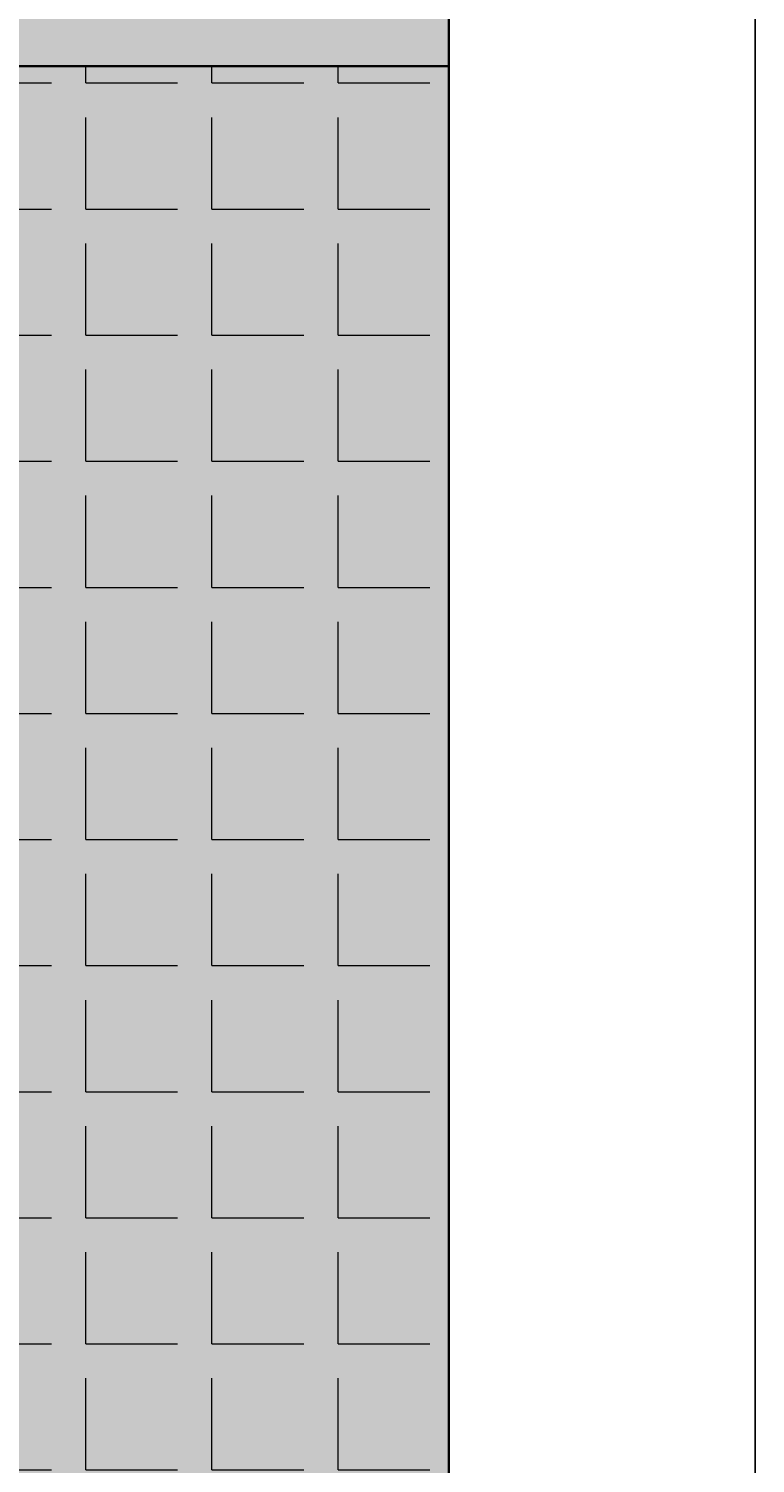
# Model space of a CAD drawing. Units: millimetres. Extents: x 1166 to 16630, y -7192 to 2820.
# Tile 4 of 8: x 7051 to 8218, y -4887 to -2583. Entities that reach past the tile are written whole.
import ezdxf

# ---------------------------------------------------------------- set-up
doc = ezdxf.new("R2010")
doc.units = ezdxf.units.MM
for name, color, linetype, lineweight in [('A-ANNO-DIMS', 2, 'Continuous', 18), ('A-FLOR-PATT', 8, 'Continuous', 13), ('A-WALL', 7, 'Continuous', 35)]:
    doc.layers.add(name, color=color, linetype=linetype, lineweight=lineweight)
doc.layers.add('A-FLOR-FNSH-PATT', color=254, linetype='Continuous', lineweight=13, true_color=0xfeeab9)
doc.layers.add('A-WALL-PATT', color=254, linetype='Continuous', lineweight=13, true_color=0xcecce6)
doc.styles.get("Standard").update_dxf_attribs({"font": 'arial.ttf'})
doc.dimstyles.get("Standard").update_dxf_attribs({"dimtxt": 0.18, "dimasz": 0.18, "dimexe": 0.18, "dimexo": 0.0625, "dimgap": 0.09, "dimtad": 0, "dimtih": 1, "dimtoh": 1, "dimdec": 4, "dimzin": 0, "dimdsep": 46, "dimtxsty": 'Standard', "dimcen": 0.09, "dimadec": 0, "dimazin": 0, "dimtfac": 1, "dimtdec": 4, "dimtofl": 0, "dimtmove": 0, "dimatfit": 3, "dimfxl": 1, "dimtolj": 1, "dimtzin": 0, "dimarcsym": 0})

# ---------------------------------------------------------------- blocks, each defined once
blk = doc.blocks.new('*D24')
at = {"layer": 'A-ANNO-DIMS', "color": 0, "lineweight": -2, "transparency": 16777216}
for p, q in [((7726.001941000004, 2327.462235000001), (8218.11944100001, 2327.462235000001)), ((8217.93944100001, 2327.282235000001), (8217.93944100001, -1988.15746197067)), ((8217.939441000011, -6303.961088000004), (8217.93944100001, -1988.521391029333)), ((7726.001941000004, -6304.141088000005), (8218.119441000012, -6304.141088000005))]:
    blk.add_line(p, q, dxfattribs=at)
at = {"layer": 'A-ANNO-DIMS', "color": 0, "transparency": 16777216}
for points in [[(8217.909441000009, 2327.282235000001), (8217.969441000008, 2327.282235000001), (8217.93944100001, 2327.462235000001)], [(8217.909441000009, -6303.961088000004), (8217.96944100001, -6303.961088000004), (8217.939441000011, -6304.141088000005)]]:
    blk.add_solid(points, dxfattribs=at)
at = {"layer": 'Defpoints', "color": 0, "transparency": 16777216}
for p in [(7725.939441000004, 2327.462235000001), (7725.939441000004, -6304.141088000005), (8217.939441000011, -6304.141088000005)]:
    blk.add_point(p, dxfattribs=at)
at = {"layer": 'A-ANNO-DIMS', "color": 0, "transparency": 16777216, "insert": (8217.939441000006, -1988.339426500003), "char_height": 0.18, "attachment_point": 5}
blk.add_mtext('\\A1;8632', dxfattribs=at)

msp = doc.modelspace()

# ---------------------------------------------------------------- hatches: boundary and pattern name
at = {"layer": 'A-FLOR-FNSH-PATT', "transparency": 33554523}
h = msp.add_hatch(color=256, dxfattribs=at)
h.dxf.hatch_style = 1
h.paths.add_polyline_path([(7725.939441137629, 2327.46223509218), (1725.939441137629, 2327.46223509218), (1725.939441137629, -5672.537764907821), (5309.614992693758, -5672.537764907821), (5309.614992693758, -2642.53776490782), (5189.614992693758, -2642.53776490782), (5189.614992693758, -5442.537764907821), (1955.939441137629, -5442.537764907819), (1955.939441137628, 2097.46223509218), (4665.939441137629, 2097.46223509218), (4665.939441137629, 150.2003357952274), (4815.939441137629, 150.2003357952271, -0.4014527144963571), (5814.98195149442, -806.0496642047723), (5815.939441137629, -806.0496642047722), (5815.939441137629, -849.7996642047723), (4815.939441137629, -849.7996642047729), (4785.939441137628, -849.7996642047729), (4785.939441137628, -902.5377649078198), (7495.939441137629, -902.5377649078199), (7495.939441137629, -2522.53776490782), (4884.014389835691, -2522.53776490782), (4884.014389835691, -2642.53776490782), (7725.939441137629, -2642.53776490782)], flags=17)
h.paths.add_polyline_path([(6066.077252941604, 618.4211469541298), (6066.077252941604, 1624.186122025141), (7407.097946088891, 1624.186122025141), (7407.097946088891, 618.4211469541295)], flags=16)
h.paths.add_polyline_path([(4979.211803565785, 660.218557639132), (4799.278299447288, 660.218557639132), (4799.278299447288, 780.1742270514636), (4789.281993662927, 790.1705328358245), (4789.281993662927, 870.1409791107119), (4799.278299447288, 880.137284895073), (4799.278299447288, 1259.996904700789), (4979.211803565785, 1259.996904700789), (4979.211803565785, 1230.007987347706), (4989.208109350147, 1230.007987347706), (4989.208109350147, 1110.052317935374), (4979.211803565785, 1110.052317935374), (4979.211803565785, 1100.056012151014), (4989.208109350147, 1100.056012151014), (4989.208109350147, 980.1003427386823), (4979.211803565785, 980.1003427386823), (4979.211803565785, 950.1114253855995), (4989.208109350147, 950.1114253855995), (4989.208109350147, 940.1151196014531, -0.0909090909092653), (4989.208109350147, 720.1963923450827), (4989.208109350147, 710.2000865609368), (4979.211803565785, 710.2000865609368)], flags=16)
h.paths.add_polyline_path([(4974.213650673605, 665.2167105313125), (4804.276452339468, 665.2167105313125), (4804.276452339468, 1254.998751808608), (4974.213650673605, 1254.998751808608)], flags=0)
h.paths.add_polyline_path([(6910.920475690947, 618.4211469541297), (6910.920475690947, 873.2148154769015), (7165.714311841242, 873.2148154769015), (7165.714311841242, 1490.084270626194), (7386.982643234919, 1490.084270626193), (7386.982643234919, 1141.419188784891), (7165.714311841242, 1141.419188784891), (7165.714311841242, 1101.188415449426), (7386.98264323492, 1101.188415449426), (7386.98264323492, 752.5231659806007), (7132.188807084624, 752.5231659806008), (7132.188807084624, 839.6893327765368)], flags=16)
h.paths.add_polyline_path([(4815.93944113763, 150.200335795227), (4665.939441137629, 150.2003357952274), (4665.939441137629, 1500.696746688973), (2460.544987272565, 1500.696746688973), (2460.544987272566, -402.5377649078198), (3575.939441137629, -402.5377649078199), (3575.93944113763, -1706.640093510054), (3463.439441137629, -1706.640093510054, 0.4014527144963571), (2714.157558370035, -2423.827593510054), (3463.439441137629, -2423.827593510054), (3463.439441137629, -2456.640093510054), (3455.939441137629, -2522.53776490782), (3455.939441137628, -2456.640093510053), (2713.439441137629, -2456.640093510054), (2713.439441137629, -2423.827593510054), (2714.157558370035, -2423.827593510054, -0.398552660000795), (3455.939441137629, -1706.6775944476), (3455.93944113763, -1706.640093510053), (3575.939441137629, -1706.640093510054), (3575.939441137629, -402.5377649078199), (2460.544987272566, -402.5377649078199), (2460.544987272565, 1500.696746688973), (4665.939441137629, 1500.696746688972), (4665.939441137629, 150.2003357952274), (4785.939441137628, 150.2003357952272), (4785.939441137628, 2097.46223509218), (7495.939441137629, 2097.46223509218), (7495.939441137629, -2522.53776490782), (4884.014389835691, -2522.53776490782), (4884.014389835691, -2642.53776490782), (7725.939441137629, -2642.53776490782), (7725.939441137629, 2327.46223509218), (1725.939441137629, 2327.46223509218), (1725.939441137629, -5672.537764907822), (5309.614992693758, -5672.53776490782), (5309.614992693758, -2642.53776490782), (4884.014389835691, -2642.53776490782), (4884.014389835691, -2522.53776490782), (4884.014389835691, -1822.53776490782), (4665.939441137629, -1822.53776490782), (4665.939441137629, -1722.53776490782), (4665.939441137629, -1022.53776490782), (4665.939441137629, -849.7996642047729), (4815.939441137629, -849.7996642047725), (4815.939441137629, -806.0496642047731), (5814.98195149442, -806.0496642047723, 0.4014527144963566)])
h.paths.add_polyline_path([(1955.939441137629, -4323.626378184433), (1965.93574692199, -4313.63007240007), (1965.93574692199, -3933.770452594356), (2145.869251040488, -3933.770452594356), (2145.869251040488, -3963.759369947439), (2155.865556824849, -3963.759369947439), (2155.865556824849, -4083.715039359769), (2145.869251040488, -4083.715039359769), (2145.869251040488, -4093.711345144131), (2155.865556824848, -4093.711345144131), (2155.865556824848, -4213.667014556462), (2145.869251040487, -4213.667014556462), (2145.869251040487, -4243.655931909545), (2155.865556824848, -4243.655931909545), (2155.865556824848, -4253.65223769369, -0.0909090909092649), (2155.865556824848, -4473.570964950059), (2155.865556824849, -4483.567270734208), (2145.869251040488, -4483.567270734208), (2145.869251040487, -4533.548799656013), (1965.935746921989, -4533.548799656013), (1965.93574692199, -4413.593130243681), (1955.939441137628, -4403.596824459319)], flags=16)
h.paths.add_polyline_path([(3017.671753088376, -1268.685150923248), (3017.671753088376, -1558.932187923503), (2092.537854326397, -1558.932187923502), (2092.537854326398, -1268.685150923248)], flags=16)
h.paths.add_polyline_path([(2768.798554444471, -687.0284595558132), (2664.903705041528, -687.0284595558132), (2696.87076529663, -782.9296403211201, -0.5013234908366285), (2617.666699633876, -1084.404517764256, -0.1328909081875925), (2584.270795046388, -1084.404517500901, -0.5013167773011727), (2505.0649162136, -782.9330743979611), (2537.033121160982, -687.0284595558132), (2489.081652205777, -687.028459555813), (2489.081652205777, -711.0041940334156), (2441.130183250573, -711.0041940334156), (2441.130183250573, -687.0284595558132), (2433.138271758039, -687.0284595558132), (2433.138271758038, -559.1578756752677), (2768.79855444447, -559.1578756752677)], flags=16)
h.paths.add_polyline_path([(2752.814731459403, -655.0608109277462, -0.4142135623730841), (2740.826866878533, -671.0446365707452), (2465.105920386106, -671.0446365707452, -0.4142135623731292), (2449.122094743107, -659.056771989874), (2449.122094743107, -591.1255243033348, -0.414213562373052), (2461.109959323975, -575.141698660336), (2736.830905816402, -575.141698660336, -0.4142135623731314), (2752.814731459403, -587.1295632412064)], flags=0)
h.paths.add_polyline_path([(2627.246667254749, -1063.015793855159, -0.2150037826741433), (2574.690827957569, -1063.015793301976, -0.4800796505542296), (2537.033991046724, -782.9313974662225), (2664.904416594217, -782.9313974662225, -0.4800795019661017)], flags=0)
h.paths.add_polyline_path([(4505.633741405676, -3647.875139181167), (4977.86337820884, -3647.875139181167, -0.190476207544349), (4977.863715650206, -5173.540873043219), (4505.633741405676, -5173.540873043219), (4505.633741405676, -5064.564758277272), (4533.929389604653, -5064.564758277272), (4533.929389604654, -3756.851253947113), (4505.633741405676, -3756.851253947113)], flags=16)
h.paths.add_polyline_path([(4880.113813381636, -4192.755706203317), (5003.372332977528, -4192.75565851188, -0.0496282101666582), (5003.372387193955, -4628.660299224469), (4880.113813381636, -4628.660251533011)], flags=0)
h.paths.add_polyline_path([(2140.871098148307, -3938.768605486535), (2140.871098148307, -4528.550646763831), (1970.933899814171, -4528.550646763831), (1970.93389981417, -3938.768605486536)], flags=0)
h.paths.add_polyline_path([(7495.939441137629, -1022.53776490782), (6660.698736718376, -1022.53776490782), (6660.698736718376, -1722.53776490782, -0.2129119084378026), (6697.901439354037, -1739.131793636166)], flags=16)
h.paths.add_polyline_path([(7495.939441137629, -1022.53776490782), (6697.901439354037, -1739.131793636166, -0.1849874276879184), (6710.698736718376, -1772.53776490782), (7495.939441137629, -1772.53776490782)], flags=16)
h.paths.add_polyline_path([(7495.939441137629, -1772.53776490782), (6710.698736718376, -1772.53776490782, -0.1849874276879184), (6697.901439354037, -1805.943736179474), (7495.939441137629, -2522.53776490782)], flags=16)
h.paths.add_polyline_path([(6697.901439354037, -1805.943736179474, -0.2129119084378014), (6660.698736718376, -1822.53776490782), (6660.698736718376, -2522.53776490782), (7495.939441137629, -2522.53776490782)], flags=16)
h.paths.add_polyline_path([(6660.698736718376, -1822.53776490782), (6438.61319335804, -1822.53776490782), (6438.61319335804, -2522.53776490782), (6660.698736718376, -2522.53776490782)], flags=16)
h.paths.add_polyline_path([(6438.61319335804, -1822.53776490782), (6216.527649997704, -1822.53776490782), (6216.527649997704, -2522.53776490782), (6438.61319335804, -2522.53776490782)], flags=16)
h.paths.add_polyline_path([(6216.527649997704, -1822.53776490782), (5994.442106637368, -1822.53776490782), (5994.442106637369, -2522.53776490782), (6216.527649997704, -2522.53776490782)], flags=16)
h.paths.add_polyline_path([(5994.442106637368, -1822.53776490782), (5772.356563277032, -1822.53776490782), (5772.356563277033, -2522.53776490782), (5994.442106637369, -2522.53776490782)], flags=16)
h.paths.add_polyline_path([(5550.271019916698, -1822.53776490782), (5328.185476556361, -1822.53776490782), (5328.185476556362, -2522.53776490782), (5550.271019916698, -2522.53776490782)], flags=16)
h.paths.add_polyline_path([(5328.185476556361, -1822.53776490782), (5106.099933196027, -1822.53776490782), (5106.099933196027, -2522.53776490782), (5328.185476556362, -2522.53776490782)], flags=16)
h.paths.add_polyline_path([(5106.099933196027, -1822.53776490782), (4884.014389835691, -1822.53776490782), (4884.014389835691, -2522.53776490782), (5106.099933196027, -2522.53776490782)], flags=16)
h.paths.add_polyline_path([(4884.014389835691, -1022.53776490782), (4665.939441137629, -1022.53776490782), (4665.939441137629, -1722.53776490782), (4884.014389835691, -1722.53776490782)], flags=16)
h.paths.add_polyline_path([(5106.099933196027, -1022.53776490782), (4884.014389835691, -1022.53776490782), (4884.014389835691, -1722.53776490782), (5106.099933196027, -1722.53776490782)], flags=16)
h.paths.add_polyline_path([(5550.271019916698, -1022.53776490782), (5328.185476556362, -1022.53776490782), (5328.185476556361, -1722.53776490782), (5550.271019916698, -1722.53776490782)], flags=16)
h.paths.add_polyline_path([(5328.185476556362, -1022.53776490782), (5106.099933196027, -1022.53776490782), (5106.099933196027, -1722.53776490782), (5328.185476556361, -1722.53776490782)], flags=16)
h.paths.add_polyline_path([(5772.356563277033, -1022.53776490782), (5550.271019916698, -1022.53776490782), (5550.271019916698, -1722.53776490782), (5772.356563277032, -1722.53776490782)], flags=16)
h.paths.add_polyline_path([(5994.442106637369, -1022.53776490782), (5772.356563277033, -1022.53776490782), (5772.356563277032, -1722.53776490782), (5994.442106637368, -1722.53776490782)], flags=16)
h.paths.add_polyline_path([(6216.527649997704, -1022.53776490782), (5994.442106637369, -1022.53776490782), (5994.442106637368, -1722.53776490782), (6216.527649997704, -1722.53776490782)], flags=16)
h.paths.add_polyline_path([(6660.698736718376, -1022.53776490782), (6438.61319335804, -1022.53776490782), (6438.61319335804, -1722.53776490782), (6660.698736718376, -1722.53776490782)], flags=16)
h.paths.add_polyline_path([(6438.61319335804, -1022.53776490782), (6216.527649997704, -1022.53776490782), (6216.527649997704, -1722.53776490782), (6438.61319335804, -1722.53776490782)], flags=16)
h.paths.add_polyline_path([(5772.356563277032, -1822.53776490782), (5550.271019916698, -1822.53776490782), (5550.271019916698, -2522.53776490782), (5772.356563277033, -2522.53776490782)], flags=16)
h.paths.add_polyline_path([(6660.698736718376, -1722.53776490782), (6438.61319335804, -1722.53776490782), (4665.939441137629, -1722.537764907819), (4665.939441137629, -1822.53776490782), (6660.698736718376, -1822.53776490782, 0.2129119084377995), (6697.901439354037, -1805.943736179474, 0.6489243663012206)], flags=16)
h.paths.add_polyline_path([(5860.250212969285, -44.00639852248207), (7154.50411478644, -44.00639852248207), (7154.50411478644, 215.6889194604054), (5860.250212969285, 215.6889194604054)], flags=24)
h.paths.add_polyline_path([(2102.335631979146, -1543.656328414819), (3007.075088498303, -1543.656328414819), (3007.075088498303, -1283.961010431932), (2102.335631979146, -1283.961010431932)], flags=8)
h.paths.add_polyline_path([(2887.503040984853, -4248.680096729577), (3740.371909930631, -4248.680096729577), (3740.371909930631, -3989.155968804687), (2887.503040984853, -3989.155968804687)], flags=24)
h.paths.add_polyline_path([(2999.435985189627, 433.0535291407016), (4111.828982060295, 433.0535291407016), (4111.828982060295, 692.5776570655913), (2999.435985189627, 692.5776570655913)], flags=24)
at = {"layer": 'A-FLOR-FNSH-PATT', "transparency": 33554590}
h = msp.add_hatch(color=256, dxfattribs=at)
h.dxf.hatch_style = 1
h.paths.add_polyline_path([(5309.614992693758, -2642.53776490782), (5309.614992693758, -6304.141088113749), (7725.939441137629, -6304.141088113749), (7725.939441137629, -5672.53776490782), (7725.939441137629, -2642.53776490782)])
edge = h.paths.add_edge_path(flags=16)
edge.add_ellipse((-448.9724108440159, -3645.429588524165), major_axis=(-7430.722679011307, 2.05049e-10), ratio=0.8423038695440578, start_angle=182.1799503136468, end_angle=183.6504275857006, ccw=False)
edge.add_line((6974.17381326888, -3362.862478220109), (6984.715647929133, -3362.862478220109))
edge.add_ellipse((6982.28108362224, -3380.396843230207), major_axis=(-20.81714882728829, 5.19e-13), ratio=0.842303869543992, start_angle=180.0000000000014, end_angle=270.0000000000014, ccw=False)
edge.add_line((7003.098232449528, -3380.396843230198), (7003.098232449528, -3722.915565549822))
edge.add_ellipse((6982.28108362224, -3720.864922613471), major_axis=(20.81714882728829, 5.097e-13), ratio=0.842303869543992, start_angle=269.9999999999985, end_angle=359.9999999999986, ccw=False)
edge.add_ellipse((-142030.922985108, -3973.064272051784), major_axis=(149013.2040687302, 7.3876543e-09), ratio=0.8423038695454406, start_angle=-0.3838667787953227, end_angle=0.09022908859151357, ccw=False)
edge.add_line((6977.567346638728, -4971.397229994678), (6984.470063297348, -4971.397229994678))
edge.add_ellipse((6982.28108362224, -4988.931595004776), major_axis=(20.81714882728829, 5.4695e-12), ratio=0.84230386954397, start_angle=-1.5006662579253316e-11, end_angle=89.99999999998488, ccw=False)
edge.add_line((7003.098232449528, -4988.931595004766), (7003.098232449527, -5331.243460438734))
edge.add_ellipse((6982.281083622239, -5329.399674388036), major_axis=(-20.81714882728829, 1.0505e-12), ratio=0.84230386954397, start_angle=90.0000000000029, end_angle=180.000000000003, ccw=False)
edge.add_line((6982.281083622243, -5346.934039398132), (6973.353954790083, -5346.934039398132))
edge.add_ellipse((-142030.922985108, -3973.064272051784), major_axis=(149013.2040687302, 7.3876543e-09), ratio=0.8423038695454406, start_angle=-0.6186431963221253, end_angle=-0.5282714718208013, ccw=False)
edge.add_ellipse((6960.189207408767, -5606.902802775503), major_axis=(-31.22572324093233, 2.0889e-12), ratio=0.8423038695439425, start_angle=179.3717627838109, end_angle=248.4647566010108, ccw=False)
edge.add_ellipse((-142041.331559525, -3973.064272085929), major_axis=(-149045.3717863939, 4.64621177404e-05), ratio=0.8423038661083152, start_angle=179.3534459208122, end_angle=179.3717628016453, ccw=False)
edge.add_ellipse((6916.869834512962, -5654.054118847628), major_axis=(-73.80201542105252, 3.6097e-12), ratio=0.8423038695439748, start_angle=90.00000000006492, end_angle=179.353445902922, ccw=False)
edge.add_line((6916.869834513031, -5716.217842016925), (5995.230132669023, -5716.217842016909))
edge.add_ellipse((5995.230132669163, -5654.054118847574), major_axis=(73.80201542109666, 3.978e-13), ratio=0.8423038695439887, start_angle=180.6465540970575, end_angle=269.9999999998622, ccw=False)
edge.add_ellipse((154953.4315273228, -3973.06427200764), major_axis=(-149045.3717871212, 2.2898328512e-06), ratio=0.8423038697262194, start_angle=0.6282372171232851, end_angle=0.6465540979564253, ccw=False)
edge.add_ellipse((5951.910759773294, -5606.902802775455), major_axis=(31.22572324094488, 4.9039e-12), ratio=0.842303869543988, start_angle=111.53524350401449, end_angle=180.6282372161637, ccw=False)
edge.add_ellipse((154943.0229527065, -3973.064272049507), major_axis=(-149013.2040691466, 7.4869171e-09), ratio=0.8423038695459824, start_angle=0.528271471820176, end_angle=0.6465540970638131, ccw=False)
edge.add_line((5938.746012391977, -5346.934039398132), (5927.384319252956, -5346.934039398132))
edge.add_ellipse((5929.818883559845, -5329.399674388033), major_axis=(20.8171488272892, 3.11e-13), ratio=0.8423038695440205, start_angle=179.9999999999992, end_angle=269.9999999999962, ccw=False)
edge.add_line((5909.001734732555, -5329.399674388034), (5909.001734732554, -4986.88095206843))
edge.add_ellipse((5929.818883559843, -4988.931595004776), major_axis=(-20.8171488272892, 3.063e-13), ratio=0.8423038695440205, start_angle=-89.99999999999608, end_angle=7.958078640513122e-13, ccw=False)
edge.add_line((5929.818883559843, -4971.397229994676), (5934.53262054336, -4971.397229994676))
edge.add_ellipse((154943.0229527065, -3973.064272049507), major_axis=(-149013.2040691466, 7.4869171e-09), ratio=0.8423038695459824, start_angle=-0.09022908859031986, end_angle=0.38386677879520903, ccw=False)
edge.add_ellipse((5929.818883559843, -3720.864922613471), major_axis=(-20.8171488272892, 1.5867e-12), ratio=0.8423038695439331, start_angle=4.376943252282217e-12, end_angle=90.00000000000438, ccw=False)
edge.add_line((5909.001734732555, -3720.864922613478), (5909.001734732555, -3378.346200293855))
edge.add_ellipse((5929.818883559843, -3380.396843230207), major_axis=(20.8171488272892, 9.396e-13), ratio=0.8423038695439548, start_angle=89.99999999999739, end_angle=179.9999999999975, ccw=False)
edge.add_line((5929.818883559843, -3362.862478220109), (5937.926153913206, -3362.862478220109))
edge.add_ellipse((13361.0723780261, -3645.42958852417), major_axis=(7430.722679011307, 7.96527e-11), ratio=0.8423038695440075, start_angle=176.3495724143003, end_angle=177.8200496863542, ccw=False)
edge.add_ellipse((6843.238962592569, -6808.26137511002), major_axis=(4407.332901654202, 4.993684e-10), ratio=0.8423038695438785, start_angle=102.12596555227748, end_angle=103.7805289894913, ccw=False)
edge.add_ellipse((6843.238962592481, -6711.831352601092), major_axis=(4294.727564406183, 8.108409e-10), ratio=0.8423038695438188, start_angle=100.20953899713243, end_angle=102.4446272934332, ccw=False)
edge.add_ellipse((5718.978043047074, -189.3416182050969), major_axis=(-3530.283493235897, 2.29487e-11), ratio=0.8423038695439934, start_angle=99.25656600720184, end_angle=102.5549326441376)
edge.add_line((6369.842688727707, -3111.939026631001), (6452.046781461999, -3066.482546539763))
edge.add_ellipse((6456.049983591043, -3074.756545497792), major_axis=(-10.40857441364578, 1.5838e-12), ratio=0.8423038695437935, start_angle=270.0000000000206, end_angle=307.9331304598557, ccw=False)
edge.add_ellipse((6456.049983591043, -3074.756545497792), major_axis=(-10.40857441364578, 1.5838e-12), ratio=0.8423038695437935, start_angle=232.06686954016618, end_angle=270.0000000000206, ccw=False)
edge.add_line((6461.762224667734, -3067.427595530816), (6542.257278454378, -3111.939026631002))
edge.add_ellipse((7193.121924135012, -189.3416182050969), major_axis=(3530.283493235459, 5.426614e-10), ratio=0.842303869544094, start_angle=257.4450673558539, end_angle=260.7434339927895)
edge.add_ellipse((6068.861004589511, -6711.831352601148), major_axis=(4294.72756440461, 7.517164e-10), ratio=0.8423038695441345, start_angle=77.55537270654469, end_angle=79.79046100284552, ccw=False)
edge.add_ellipse((6068.86100458951, -6808.26137511002), major_axis=(-4407.332901654327, 6.637773e-10), ratio=0.842303869543856, start_angle=256.2194710105107, end_angle=257.8740344477245, ccw=False)
edge = h.paths.add_edge_path(flags=0)
edge.add_ellipse((5799.636342679871, -3484.80630294614), major_axis=(790.1331889300527, 2.1537e-12), ratio=0.8423038695439757, start_angle=-2.2737367544323206e-13, end_angle=29.43856959797921, ccw=False)
edge.add_line((6589.769531609924, -3484.806302946152), (6589.769531609924, -3517.865771969153))
edge.add_line((6589.769531609924, -3517.865771969153), (6615.396946753699, -3517.865771969153))
edge.add_ellipse((6612.950235160742, -3526.632954474201), major_axis=(10.40857441364348, 1.5653e-12), ratio=0.8423038695440233, start_angle=45.51978911742219, end_angle=89.99999999999147, ccw=False)
edge.add_line((6619.58436781158, -3519.877346340421), (6697.576744801804, -3574.216072032502))
edge.add_line((6697.576744801804, -3574.216072032502), (6697.576744801804, -3782.552340767745))
edge.add_ellipse((6643.673138205864, -3780.461483581003), major_axis=(5.016450041930374, 89.18653102701357), ratio=0.6038335755719256, start_angle=106.34259195429391, end_angle=270.99798572497, ccw=False)
edge.add_line((6589.769531609924, -3793.028339937766), (6589.769531609924, -3484.806302946153))
edge.add_ellipse((5799.636342679871, -3484.80630294614), major_axis=(790.1331889300527, 2.1537e-12), ratio=0.8423038695439757, start_angle=-2.143e-13, end_angle=29.43856959797918)
edge.add_ellipse((7112.463624502211, -3484.80630294614), major_axis=(-790.1331889300524, 7.9434e-12), ratio=0.8423038695439707, start_angle=-29.43856959797882, end_angle=5.465e-13)
edge.add_line((6322.330435572158, -3484.806302946151), (6322.330435572158, -3793.028339937766))
edge.add_ellipse((6268.426828976219, -3780.461483581003), major_axis=(-5.016450041930374, 89.18653102701357), ratio=0.6038335755719256, start_angle=89.00201427502998, end_angle=253.6574080457062, ccw=False)
edge.add_line((6214.523222380278, -3782.552340767737), (6214.523222380279, -3574.216072032502))
edge.add_line((6214.523222380279, -3574.216072032502), (6294.400928520307, -3518.563802793423))
edge.add_ellipse((6299.149732021341, -3526.632954474201), major_axis=(10.4085744136453, 3.381e-13), ratio=0.8423038695438764, start_angle=89.9999999999983, end_angle=134.4802108825654, ccw=False)
edge.add_line((6299.149732021338, -3517.865771969152), (6322.330435572158, -3517.865771969152))
edge.add_line((6322.330435572158, -3517.865771969152), (6322.330435572158, -3484.806302946154))
edge.add_ellipse((7112.463624502211, -3484.80630294614), major_axis=(-790.1331889300524, 7.9434e-12), ratio=0.8423038695439707, start_angle=-29.438569597978812, end_angle=6.252776074688882e-13, ccw=False)
edge = h.paths.add_edge_path(flags=0)
edge.add_line((6899.672020630411, -4051.112638739672), (6868.937058315451, -4281.473694083312))
edge.add_ellipse((6495.430033257824, -5170.362894493258), major_axis=(1119.455420763322, 3.0514e-12), ratio=0.8423038695439744, start_angle=67.20808512240981, end_angle=85.12993040286408)
edge.add_line((6575.564661792019, -4229.860228440724), (6336.53530539007, -4229.860228440724))
edge.add_ellipse((6416.669933924288, -5170.362894493482), major_axis=(1119.455420763633, 5.82337e-11), ratio=0.842303869543943, start_angle=94.87006959713275, end_angle=112.7919148775836)
edge.add_line((6043.162908866626, -4281.473694083309), (6012.427946551666, -4051.112638739666))
edge.add_ellipse((6380.264280565288, -4969.144446445703), major_axis=(1150.303461305961, 5.9583e-11), ratio=0.8423038695439412, start_angle=94.27742096305099, end_angle=111.83495379670521, ccw=False)
edge.add_line((6307.939299228742, -4002.156437400477), (6604.160667953341, -4002.156437400477))
edge.add_ellipse((6531.835686616772, -4969.144446445682), major_axis=(-1150.303461305901, 2.25473e-11), ratio=0.8423038695439672, start_angle=248.1650462032914, end_angle=265.72257903694555, ccw=False)
edge = h.paths.add_edge_path(flags=0)
edge.add_ellipse((-142030.9229855244, -3973.064272050007), major_axis=(-148992.3869203194, 2.076209e-10), ratio=0.842303869544003, start_angle=179.6222358060902, end_angle=179.9444056865007, ccw=False)
edge.add_line((6956.899516505626, -4955.389335168179), (6903.06848209712, -4744.029778632651))
edge.add_ellipse((-45118.92430422086, -4413.460367112857), major_axis=(52023.47313689829, 7.771381e-10), ratio=0.842303869543516, start_angle=-0.3640763488911976, end_angle=0.1208973690317991)
edge.add_line((6904.3855953652, -4303.688047353878), (6961.365076797346, -4117.63210307358))
edge = h.paths.add_edge_path(flags=0)
edge.add_line((5950.734890384741, -4117.632103073563), (6007.714371816899, -4303.688047353918))
edge.add_ellipse((58031.02427140294, -4413.460367113082), major_axis=(-52023.47313689826, 1.3200601e-09), ratio=0.8423038695497072, start_angle=-0.1208973690315197, end_angle=0.364076348891516)
edge.add_line((6009.031485084967, -4744.029778632643), (5955.200450676423, -4955.389335168309))
edge.add_ellipse((154943.0229527063, -3973.064272050686), major_axis=(-148992.3869203192, 3.28274152e-08), ratio=0.8423038695536886, start_angle=0.05559431351167632, end_angle=0.3777641939223031, ccw=False)
edge = h.paths.add_edge_path(flags=0)
edge.add_line((6868.937058315452, -5013.198477251068), (6868.937058315452, -5277.993200767081))
edge.add_ellipse((6456.049983591043, -3571.079447459644), major_axis=(2068.11644385622, 7.9333e-12), ratio=0.8423038695439821, start_angle=256.4018653097692, end_angle=283.59813469023027, ccw=False)
edge.add_line((6043.16290886663, -5277.993200767081), (6043.16290886663, -5013.198477251068))
edge.add_ellipse((6456.049983591043, -3306.284723943631), major_axis=(2068.116443856253, 3.3411e-12), ratio=0.8423038695439679, start_angle=256.4018653097692, end_angle=283.5981346902304)
edge = h.paths.add_edge_path(flags=0)
edge.add_ellipse((6827.302760660877, -5415.313265203762), major_axis=(-41.63429765457658, 1.038e-12), ratio=0.842303869543992, start_angle=180.0000000000014, end_angle=270.0000000000014, ccw=False)
edge.add_line((6868.937058315454, -5415.313265203762), (6868.937058315454, -5689.12284886784))
edge.add_line((6868.937058315454, -5689.12284886784), (6043.162908866631, -5689.122848867824))
edge.add_line((6043.162908866631, -5689.122848867824), (6043.16290886663, -5415.313265203758))
edge.add_ellipse((6084.797206521206, -5415.313265203759), major_axis=(-41.63429765457658, 3.4138e-12), ratio=0.842303869543992, start_angle=-89.99999999999523, end_angle=4.718003765447065e-12, ccw=False)
edge.add_line((6084.797206521207, -5380.244535183563), (6827.302760660879, -5380.244535183566))
h.paths.add_polyline_path([(3455.939441137629, -522.53776490782), (1955.939441137629, -522.53776490782), (1955.939441137629, -2522.53776490782), (3455.939441137629, -2522.53776490782), (3455.939441137628, -2456.640093510054), (2713.439441137629, -2456.640093510054), (2713.43944113763, -2423.827593510054), (2714.157558370035, -2423.827593510054, -0.398552660000795), (3455.939441137629, -1706.6775944476)])
h.paths.add_polyline_path([(2617.666699633915, -1084.404517764245, -0.1328909081885223), (2584.2707950462, -1084.404517500826, -0.5013167773008519), (2505.064916213601, -782.9330743979599), (2537.033121160981, -687.0284595558127), (2489.081652205778, -687.0284595558132), (2489.081652205778, -711.0041940334158), (2441.130183250573, -711.0041940334158), (2441.130183250573, -695.0203710483474), (2473.097829220709, -695.0203710483474), (2473.097829220709, -687.0284595558132), (2433.13827175804, -687.0284595558132), (2433.138271758038, -559.1578756752674), (2768.79855444447, -559.1578756752674), (2768.798554444471, -687.0284595558132), (2664.903705041528, -687.0284595558132), (2696.870765296628, -782.9296403211174, -0.5013234908365807)], flags=16)
h.paths.add_polyline_path([(2627.246667254758, -1063.015793855155, -0.2150037826753064), (2574.690827957319, -1063.015793301825, -0.4800796505537303), (2537.033991046725, -782.9313974662227), (2664.904416594217, -782.9313974662227, -0.4800795019660876)], flags=0)
h.paths.add_polyline_path([(2736.830905816404, -671.0446365707452), (2465.105920386107, -671.0446365707452, -0.5000001164022092), (2449.122094743107, -655.0608109277463), (2449.122094743107, -591.1255243033341, -0.5000001164022404), (2465.105920386111, -575.1416986603361), (2736.830905816402, -575.1416986603361, -0.5000001164023353), (2752.814731459403, -591.1255243033406), (2752.814731459403, -655.0608109277468, -0.50000011640211)], flags=0)
h.paths.add_polyline_path([(5931.781743219382, -6111.826019846759), (7070.309755611069, -6111.826019846759), (7070.309755611069, -5852.301891921869), (5931.781743219382, -5852.301891921869)], flags=24)
h.paths.add_polyline_path([(2102.335631979146, -1543.656328414819), (3007.075088498303, -1543.656328414819), (3007.075088498303, -1283.961010431932), (2102.335631979146, -1283.961010431932)], flags=24)
at = {"layer": 'A-FLOR-PATT', "transparency": 33554564}
h = msp.add_hatch(dxfattribs=at)
h.set_pattern_fill('ANGLE', color=256, scale=29)
h.set_pattern_definition([(0, (-8657.519420588213, -11987.85165359825), (0, 202.565), [147.32, -55.24499999999999]), (90, (-8657.519420588213, -11987.85165359825), (-202.565, 1.24e-14), [147.32, -55.24499999999999])])
h.paths.add_polyline_path([(7725.939441137629, -2642.53776490782), (5309.614992693758, -2642.53776490782), (5309.614992693758, -6304.141088113749), (7725.939441137629, -6304.141088113749), (7725.939441137629, -5672.53776490782)])
edge = h.paths.add_edge_path(flags=16)
edge.add_ellipse((-142030.922985108, -3973.064272051784), major_axis=(149013.2040687302, 7.3876543e-09), ratio=0.8423038695454406, start_angle=-0.3838667787953227, end_angle=0.09022908859151357, ccw=False)
edge.add_ellipse((6982.28108362224, -4988.931595004776), major_axis=(20.81714882728829, 5.4695e-12), ratio=0.84230386954397, start_angle=-1.5006662579253316e-11, end_angle=89.99999999998488, ccw=False)
edge.add_line((7003.098232449528, -4988.931595004773), (7003.098232449527, -5329.399674388036))
edge.add_ellipse((6982.281083622239, -5329.399674388036), major_axis=(-20.81714882728829, 1.0505e-12), ratio=0.84230386954397, start_angle=90.0000000000029, end_angle=180.000000000003, ccw=False)
edge.add_line((6982.281083622241, -5346.934039398132), (6973.353954790083, -5346.934039398132))
edge.add_ellipse((-142030.922985108, -3973.064272051784), major_axis=(149013.2040687302, 7.3876543e-09), ratio=0.8423038695454406, start_angle=-0.6186431963221253, end_angle=-0.5282714718208013, ccw=False)
edge.add_ellipse((6960.189207408767, -5606.902802775503), major_axis=(-31.22572324093233, 2.0889e-12), ratio=0.8423038695439425, start_angle=179.3717627838109, end_angle=248.4647566010108, ccw=False)
edge.add_ellipse((-142041.331559525, -3973.064272085929), major_axis=(-149045.3717863939, 4.64621177404e-05), ratio=0.8423038661083152, start_angle=179.3534459208122, end_angle=179.3717628016453, ccw=False)
edge.add_ellipse((6916.869834512962, -5654.054118847628), major_axis=(-73.80201542105252, 3.6097e-12), ratio=0.8423038695439748, start_angle=90.00000000006492, end_angle=179.353445902922, ccw=False)
edge.add_line((6916.869834513029, -5716.217842016925), (5995.230132669016, -5716.217842016909))
edge.add_ellipse((5995.230132669163, -5654.054118847574), major_axis=(73.80201542109666, 3.978e-13), ratio=0.8423038695439887, start_angle=180.6465540970575, end_angle=269.9999999998622, ccw=False)
edge.add_ellipse((154953.4315273228, -3973.06427200764), major_axis=(-149045.3717871212, 2.2898328512e-06), ratio=0.8423038697262194, start_angle=0.6282372171232851, end_angle=0.6465540979564253, ccw=False)
edge.add_ellipse((5951.910759773294, -5606.902802775455), major_axis=(31.22572324094488, 4.9039e-12), ratio=0.842303869543988, start_angle=111.53524350401449, end_angle=180.6282372161637, ccw=False)
edge.add_ellipse((154943.0229527065, -3973.064272049507), major_axis=(-149013.2040691466, 7.4869171e-09), ratio=0.8423038695459824, start_angle=0.528271471820176, end_angle=0.6465540970638131, ccw=False)
edge.add_line((5938.746012391977, -5346.934039398132), (5929.818883559843, -5346.934039398132))
edge.add_ellipse((5929.818883559845, -5329.399674388033), major_axis=(20.8171488272892, 3.11e-13), ratio=0.8423038695440205, start_angle=179.9999999999992, end_angle=269.9999999999962, ccw=False)
edge.add_line((5909.001734732555, -5329.399674388033), (5909.001734732554, -4988.931595004778))
edge.add_ellipse((5929.818883559843, -4988.931595004776), major_axis=(-20.8171488272892, 3.063e-13), ratio=0.8423038695440205, start_angle=-89.99999999999608, end_angle=7.958078640513122e-13, ccw=False)
edge.add_ellipse((154943.0229527065, -3973.064272049507), major_axis=(-149013.2040691466, 7.4869171e-09), ratio=0.8423038695459824, start_angle=-0.09022908859031986, end_angle=0.38386677879520903, ccw=False)
edge.add_ellipse((5929.818883559843, -3720.864922613471), major_axis=(-20.8171488272892, 1.5867e-12), ratio=0.8423038695439331, start_angle=4.376943252282217e-12, end_angle=90.00000000000438, ccw=False)
edge.add_line((5909.001734732555, -3720.864922613472), (5909.001734732555, -3380.396843230204))
edge.add_ellipse((5929.818883559843, -3380.396843230207), major_axis=(20.8171488272892, 9.396e-13), ratio=0.8423038695439548, start_angle=89.99999999999739, end_angle=179.9999999999975, ccw=False)
edge.add_line((5929.818883559843, -3362.862478220109), (5937.926153913207, -3362.862478220109))
edge.add_ellipse((13361.0723780261, -3645.42958852417), major_axis=(7430.722679011307, 7.96527e-11), ratio=0.8423038695440075, start_angle=176.3495724143003, end_angle=177.8200496863542, ccw=False)
edge.add_ellipse((6843.238962592569, -6808.26137511002), major_axis=(4407.332901654202, 4.993684e-10), ratio=0.8423038695438785, start_angle=102.12596555227748, end_angle=103.7805289894913, ccw=False)
edge.add_ellipse((6843.238962592481, -6711.831352601092), major_axis=(4294.727564406183, 8.108409e-10), ratio=0.8423038695438188, start_angle=100.20953899713243, end_angle=102.4446272934332, ccw=False)
edge.add_ellipse((5718.978043047074, -189.3416182050969), major_axis=(-3530.283493235897, 2.29487e-11), ratio=0.8423038695439934, start_angle=99.25656600720184, end_angle=102.5549326441376)
edge.add_line((6369.842688727707, -3111.939026631), (6453.505541262713, -3065.675894661087))
edge.add_ellipse((6456.049983591043, -3074.756545497792), major_axis=(-10.40857441364578, 1.5838e-12), ratio=0.8423038695437935, start_angle=232.06686954016618, end_angle=270.0000000000206, ccw=False)
edge.add_line((6460.053185720086, -3066.482546539763), (6542.257278454378, -3111.939026631002))
edge.add_ellipse((7193.121924135012, -189.3416182050969), major_axis=(3530.283493235459, 5.426614e-10), ratio=0.842303869544094, start_angle=257.4450673558539, end_angle=260.7434339927895)
edge.add_ellipse((6068.861004589511, -6711.831352601148), major_axis=(4294.72756440461, 7.517164e-10), ratio=0.8423038695441345, start_angle=77.55537270654469, end_angle=79.79046100284552, ccw=False)
edge.add_ellipse((6068.86100458951, -6808.26137511002), major_axis=(-4407.332901654327, 6.637773e-10), ratio=0.842303869543856, start_angle=256.2194710105107, end_angle=257.8740344477245, ccw=False)
edge.add_ellipse((-448.9724108440159, -3645.429588524165), major_axis=(-7430.722679011307, 2.05049e-10), ratio=0.8423038695440578, start_angle=182.1799503136468, end_angle=183.6504275857006, ccw=False)
edge.add_line((6974.17381326888, -3362.862478220109), (6982.28108362224, -3362.862478220109))
edge.add_ellipse((6982.28108362224, -3380.396843230207), major_axis=(-20.81714882728829, 5.19e-13), ratio=0.842303869543992, start_angle=180.0000000000014, end_angle=270.0000000000014, ccw=False)
edge.add_line((7003.098232449528, -3380.396843230204), (7003.098232449528, -3720.864922613474))
edge.add_ellipse((6982.28108362224, -3720.864922613471), major_axis=(20.81714882728829, 5.097e-13), ratio=0.842303869543992, start_angle=269.9999999999985, end_angle=359.9999999999986, ccw=False)
edge = h.paths.add_edge_path(flags=0)
edge.add_ellipse((-142030.9229855244, -3973.064272050007), major_axis=(-148992.3869203194, 2.076209e-10), ratio=0.842303869544003, start_angle=179.6222358060902, end_angle=179.9444056865007, ccw=False)
edge.add_line((6956.899516505626, -4955.389335168179), (6903.06848209712, -4744.029778632651))
edge.add_ellipse((-45118.92430422086, -4413.460367112857), major_axis=(52023.47313689829, 7.771381e-10), ratio=0.842303869543516, start_angle=-0.3640763488911976, end_angle=0.1208973690317991)
edge.add_line((6904.3855953652, -4303.688047353878), (6961.365076797346, -4117.632103073563))
edge = h.paths.add_edge_path(flags=0)
edge.add_line((6899.672020630411, -4051.112638739673), (6868.937058315451, -4281.473694083312))
edge.add_ellipse((6495.430033257824, -5170.362894493258), major_axis=(1119.455420763322, 3.0514e-12), ratio=0.8423038695439744, start_angle=67.20808512240981, end_angle=85.12993040286408)
edge.add_line((6575.564661792022, -4229.860228440724), (6336.535305390071, -4229.860228440724))
edge.add_ellipse((6416.669933924288, -5170.362894493482), major_axis=(1119.455420763633, 5.82337e-11), ratio=0.842303869543943, start_angle=94.87006959713275, end_angle=112.7919148775836)
edge.add_line((6043.162908866626, -4281.473694083308), (6012.427946551666, -4051.112638739666))
edge.add_ellipse((6380.264280565288, -4969.144446445703), major_axis=(1150.303461305961, 5.9583e-11), ratio=0.8423038695439412, start_angle=94.27742096305099, end_angle=111.83495379670521, ccw=False)
edge.add_line((6307.939299228742, -4002.156437400477), (6604.16066795334, -4002.156437400477))
edge.add_ellipse((6531.835686616772, -4969.144446445682), major_axis=(-1150.303461305901, 2.25473e-11), ratio=0.8423038695439672, start_angle=248.1650462032914, end_angle=265.72257903694555, ccw=False)
edge = h.paths.add_edge_path(flags=0)
edge.add_ellipse((6643.673138205864, -3780.461483581003), major_axis=(5.016450041930374, 89.18653102701357), ratio=0.6038335755719256, start_angle=106.34259195429391, end_angle=270.99798572497, ccw=False)
edge.add_line((6589.769531609924, -3793.028339937766), (6589.769531609924, -3484.806302946154))
edge.add_ellipse((5799.636342679871, -3484.80630294614), major_axis=(790.1331889300527, 2.1537e-12), ratio=0.8423038695439757, start_angle=-2.143e-13, end_angle=29.43856959797918)
edge.add_ellipse((7112.463624502211, -3484.80630294614), major_axis=(-790.1331889300524, 7.9434e-12), ratio=0.8423038695439707, start_angle=-29.43856959797882, end_angle=5.465e-13)
edge.add_line((6322.330435572158, -3484.806302946151), (6322.330435572158, -3793.028339937766))
edge.add_ellipse((6268.426828976219, -3780.461483581003), major_axis=(-5.016450041930374, 89.18653102701357), ratio=0.6038335755719256, start_angle=89.00201427502998, end_angle=253.6574080457062, ccw=False)
edge.add_line((6214.523222380278, -3782.552340767735), (6214.523222380279, -3574.216072032502))
edge.add_line((6214.523222380279, -3574.216072032502), (6295.402812213822, -3517.865771969152))
edge.add_line((6295.402812213822, -3517.865771969152), (6322.330435572158, -3517.865771969152))
edge.add_line((6322.330435572158, -3517.865771969152), (6322.330435572158, -3484.806302946154))
edge.add_ellipse((7112.463624502211, -3484.80630294614), major_axis=(-790.1331889300524, 7.9434e-12), ratio=0.8423038695439707, start_angle=-29.438569597978812, end_angle=6.252776074688882e-13, ccw=False)
edge.add_ellipse((5799.636342679871, -3484.80630294614), major_axis=(790.1331889300527, 2.1537e-12), ratio=0.8423038695439757, start_angle=-2.2737367544323206e-13, end_angle=29.43856959797921, ccw=False)
edge.add_line((6589.769531609924, -3484.806302946153), (6589.769531609924, -3517.865771969153))
edge.add_line((6589.769531609924, -3517.865771969153), (6616.697154968261, -3517.865771969153))
edge.add_line((6616.697154968261, -3517.865771969153), (6697.576744801804, -3574.216072032502))
edge.add_line((6697.576744801804, -3574.216072032502), (6697.576744801804, -3782.552340767746))
edge = h.paths.add_edge_path(flags=0)
edge.add_line((6868.937058315452, -5013.198477251068), (6868.937058315452, -5277.993200767081))
edge.add_ellipse((6456.049983591043, -3571.079447459644), major_axis=(2068.11644385622, 7.9333e-12), ratio=0.8423038695439821, start_angle=256.4018653097692, end_angle=283.59813469023027, ccw=False)
edge.add_line((6043.16290886663, -5277.993200767081), (6043.16290886663, -5013.198477251067))
edge.add_ellipse((6456.049983591043, -3306.284723943631), major_axis=(2068.116443856253, 3.3411e-12), ratio=0.8423038695439679, start_angle=256.4018653097692, end_angle=283.5981346902304)
edge = h.paths.add_edge_path(flags=0)
edge.add_ellipse((58031.02427140294, -4413.460367113082), major_axis=(-52023.47313689826, 1.3200601e-09), ratio=0.8423038695497072, start_angle=-0.1208973690315197, end_angle=0.364076348891516)
edge.add_line((6009.031485084967, -4744.029778632643), (5955.200450676423, -4955.389335168309))
edge.add_ellipse((154943.0229527063, -3973.064272050686), major_axis=(-148992.3869203192, 3.28274152e-08), ratio=0.8423038695536886, start_angle=0.05559431351167632, end_angle=0.3777641939223031, ccw=False)
edge.add_line((5950.734890384742, -4117.632103073569), (6007.714371816899, -4303.688047353918))
edge = h.paths.add_edge_path(flags=0)
edge.add_ellipse((6827.302760660877, -5415.313265203762), major_axis=(-41.63429765457658, 1.038e-12), ratio=0.842303869543992, start_angle=180.0000000000014, end_angle=270.0000000000014, ccw=False)
edge.add_line((6868.937058315454, -5415.313265203762), (6868.937058315454, -5689.12284886784))
edge.add_line((6868.937058315454, -5689.12284886784), (6043.162908866631, -5689.122848867824))
edge.add_line((6043.162908866631, -5689.122848867824), (6043.16290886663, -5415.31326520376))
edge.add_ellipse((6084.797206521206, -5415.313265203759), major_axis=(-41.63429765457658, 3.4138e-12), ratio=0.842303869543992, start_angle=-89.99999999999523, end_angle=4.718003765447065e-12, ccw=False)
edge.add_line((6084.797206521206, -5380.244535183563), (6827.302760660877, -5380.244535183566))
at = {"layer": 'A-WALL-PATT'}
h = msp.add_hatch(color=256, dxfattribs=at)
h.dxf.hatch_style = 1
h.paths.add_polyline_path([(1955.939441137629, 2097.46223509218), (4665.939441137629, 2097.46223509218), (4665.939441137629, 150.2003357952274), (4785.939441137628, 150.2003357952273), (4785.939441137628, 2097.46223509218), (7495.939441137629, 2097.46223509218), (7495.939441137629, -2522.53776490782), (4884.014389835691, -2522.53776490782), (4884.014389835691, -2642.53776490782), (7725.939441137629, -2642.53776490782), (7725.93944113763, 2327.46223509218), (1725.939441137629, 2327.46223509218), (1725.939441137629, -5672.537764907819), (5309.614992693758, -5672.537764907821), (5309.614992693758, -2642.53776490782), (5189.614992693758, -2642.53776490782), (5189.614992693758, -5442.53776490782), (1955.939441137629, -5442.53776490782)])
h.paths.add_polyline_path([(7495.939441137629, -902.5377649078199), (4785.939441137628, -902.5377649078199), (4785.939441137628, -849.7996642047729), (4665.939441137629, -849.7996642047729), (4665.939441137629, -1022.53776490782), (7495.939441137629, -1022.53776490782)], flags=17)
h.paths.add_polyline_path([(3575.939441137629, -402.5377649078199), (1955.939441137629, -402.5377649078199), (1955.939441137629, -522.53776490782), (3455.939441137629, -522.5377649078201), (3455.939441137629, -1706.640093510054), (3575.939441137629, -1706.640093510054)], flags=17)
h.paths.add_polyline_path([(3575.939441137629, -2456.640093510053), (3455.939441137629, -2456.640093510054), (3455.939441137629, -2522.53776490782), (1955.939441137629, -2522.53776490782), (1955.939441137629, -2642.53776490782), (3575.939441137629, -2642.53776490782)], flags=17)

# ---------------------------------------------------------------- linework, layer by layer
at = {"layer": 'A-WALL'}
msp.add_line((4884.014389835691, -2642.53776490782), (7725.939441137629, -2642.53776490782), dxfattribs=at)
msp.add_lwpolyline([(5309.614992693758, -5672.53776490782), (1725.939441137629, -5672.53776490782), (1725.939441137629, 2327.46223509218), (7725.939441137629, 2327.46223509218), (7725.939441137629, -5672.53776490782)], dxfattribs=at)

# ---------------------------------------------------------------- dimensions: what is measured, and where the dimension line sits
at = {"layer": 'A-ANNO-DIMS'}
dim = msp.add_linear_dim(base=(8217.939441000011, -6304.141088000005), p1=(7725.939441000001, 2327.462235), p2=(7725.939441000001, -6304.141088000001), angle=90, dimstyle='Standard', override={"dimdec": 0, "dimlfac": 1, "dimrnd": 0, "dimzin": 0, "dimdsep": 46, "dimlunit": 2}, dxfattribs=at)
dim.commit()
dim.dimension.update_dxf_attribs({"geometry": '*D24', "text_midpoint": (8217.939441000006, -1988.339426500003)})

doc.saveas('drawing.dxf')
